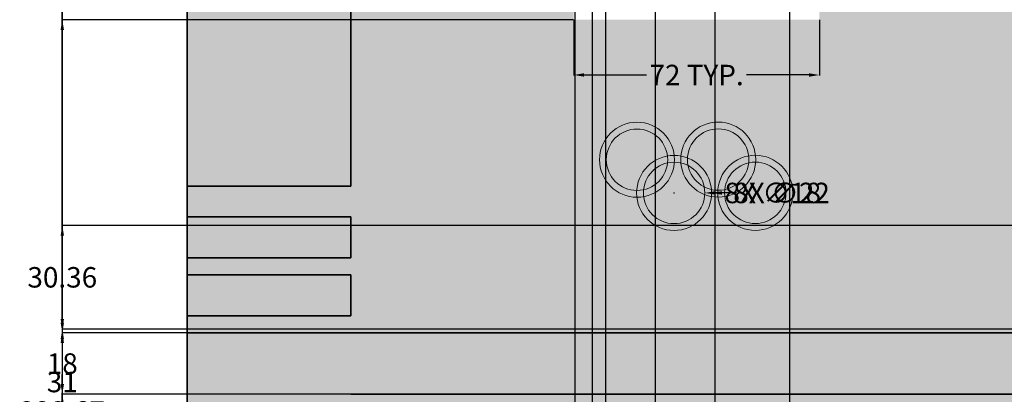
# Model space of a CAD drawing. Units: inches. Extents: x 126 to 726, y 86 to 888.
# Tile 7 of 13: x 137 to 426, y 546 to 655. Entities that reach past the tile are written whole.
import ezdxf

# ---------------------------------------------------------------- set-up
doc = ezdxf.new("R2010")
doc.units = ezdxf.units.IN
doc.header["$MEASUREMENT"] = 0
for name, color, linetype, lineweight in [('A-ANNO-DIMS', 2, 'Continuous', 18), ('A-ELEV', 7, 'Continuous', 35), ('A-ELEV-DECO', 7, 'Continuous', 18), ('A-ELEV-PATT', 8, 'Continuous', 13)]:
    doc.layers.add(name, color=color, linetype=linetype, lineweight=lineweight)
doc.styles.get("Standard").update_dxf_attribs({"font": 'arial.ttf'})
doc.dimstyles.get("Standard").update_dxf_attribs({"dimtxt": 6, "dimasz": 3, "dimexe": 0.18, "dimexo": 0.0625, "dimgap": 0.09, "dimtad": 0, "dimtih": 1, "dimtoh": 1, "dimdec": 0, "dimzin": 0, "dimdsep": 46, "dimlunit": 3, "dimtxsty": 'Standard', "dimcen": 0.09, "dimadec": 0, "dimazin": 0, "dimtfac": 1, "dimtdec": 0, "dimtofl": 0, "dimtmove": 0, "dimatfit": 3, "dimfxl": 1, "dimtolj": 1, "dimtzin": 0, "dimarcsym": 0})

# ---------------------------------------------------------------- blocks, each defined once
blk = doc.blocks.new('FACADE-STRIP')
for p, q in [((0, 0), (0, 12)), ((0, 12), (48, 12)), ((0, 0), (48, 0))]:
    blk.add_line(p, q)
blk = doc.blocks.new('MOTIF-RINGS')
for centre, radius in [((34.81, 20.77), 11), ((11, 20.74), 11), ((11, 20.74), 9), ((34.81, 20.77), 9), ((21.88, 11), 11), ((45.69, 11.03), 11), ((21.88, 11), 9), ((45.69, 11.03), 9)]:
    blk.add_circle(centre, radius)
blk = doc.blocks.new('*D6')
at = {"layer": 'A-ANNO-DIMS', "color": 0, "lineweight": -2, "transparency": 16777216}
for p, q in [((299.32, 655.29), (299.32, 638.97)), ((371.32, 655.29), (371.32, 638.97)), ((302.32, 639.15), (320.65, 639.15)), ((368.32, 639.15), (349.99, 639.15))]:
    blk.add_line(p, q, dxfattribs=at)
at = {"layer": 'A-ANNO-DIMS', "color": 0, "transparency": 16777216}
for points in [[(302.32, 639.65), (302.32, 638.65), (299.32, 639.15)], [(368.32, 639.65), (368.32, 638.65), (371.32, 639.15)]]:
    blk.add_solid(points, dxfattribs=at)
at = {"layer": 'Defpoints', "color": 0, "transparency": 16777216}
for p in [(299.32, 655.35), (371.32, 655.35), (371.32, 639.15)]:
    blk.add_point(p, dxfattribs=at)
at = {"layer": 'A-ANNO-DIMS', "color": 0, "transparency": 16777216, "insert": (335.32, 639.15), "char_height": 6, "attachment_point": 5}
blk.add_mtext('\\A1;72 TYP.', dxfattribs=at)
blk = doc.blocks.new('*D13')
at = {"layer": 'A-ANNO-DIMS', "color": 0, "lineweight": -2, "transparency": 16777216}
for p, q in [((665.97, 642.98), (665.97, 90.21)), ((185.97, 126.98), (185.97, 90.21)), ((188.97, 90.39), (419.15, 90.39)), ((662.97, 90.39), (432.8, 90.39))]:
    blk.add_line(p, q, dxfattribs=at)
at = {"layer": 'A-ANNO-DIMS', "color": 0, "transparency": 16777216}
for points in [[(188.97, 90.89), (188.97, 89.89), (185.97, 90.39)], [(662.97, 90.89), (662.97, 89.89), (665.97, 90.39)]]:
    blk.add_solid(points, dxfattribs=at)
at = {"layer": 'Defpoints', "color": 0, "transparency": 16777216}
for p in [(665.97, 643.04), (185.97, 127.04), (665.97, 90.39)]:
    blk.add_point(p, dxfattribs=at)
at = {"layer": 'A-ANNO-DIMS', "color": 0, "transparency": 16777216, "insert": (425.97, 90.39), "char_height": 6, "attachment_point": 5}
blk.add_mtext('\\A1;480', dxfattribs=at)
blk = doc.blocks.new('*D14')
at = {"layer": 'A-ANNO-DIMS', "color": 0, "lineweight": -2, "transparency": 16777216}
for p, q in [((185.91, 847.04), (149.14, 847.04)), ((149.32, 844.04), (149.32, 490.2)), ((149.32, 130.04), (149.32, 483.89)), ((185.91, 127.04), (149.14, 127.04))]:
    blk.add_line(p, q, dxfattribs=at)
at = {"layer": 'A-ANNO-DIMS', "color": 0, "transparency": 16777216}
for points in [[(148.82, 844.04), (149.82, 844.04), (149.32, 847.04)], [(148.82, 130.04), (149.82, 130.04), (149.32, 127.04)]]:
    blk.add_solid(points, dxfattribs=at)
at = {"layer": 'Defpoints', "color": 0, "transparency": 16777216}
for p in [(149.32, 847.04), (185.97, 847.04), (185.97, 127.04)]:
    blk.add_point(p, dxfattribs=at)
at = {"layer": 'A-ANNO-DIMS', "color": 0, "transparency": 16777216, "insert": (149.32, 487.04), "char_height": 6, "attachment_point": 5}
blk.add_mtext('\\A1;720', dxfattribs=at)
blk = doc.blocks.new('*D17')
at = {"layer": 'A-ANNO-DIMS', "color": 0, "lineweight": -2, "transparency": 16777216}
for p, q in [((299.26, 655.35), (149.14, 655.35)), ((149.32, 652.35), (149.32, 543.67)), ((149.32, 428.68), (149.32, 537.37)), ((299.6, 425.68), (149.14, 425.68))]:
    blk.add_line(p, q, dxfattribs=at)
at = {"layer": 'A-ANNO-DIMS', "color": 0, "transparency": 16777216}
for points in [[(148.82, 652.35), (149.82, 652.35), (149.32, 655.35)], [(148.82, 428.68), (149.82, 428.68), (149.32, 425.68)]]:
    blk.add_solid(points, dxfattribs=at)
at = {"layer": 'Defpoints', "color": 0, "transparency": 16777216}
for p in [(149.32, 655.35), (299.32, 655.35), (299.67, 425.68)]:
    blk.add_point(p, dxfattribs=at)
at = {"layer": 'A-ANNO-DIMS', "color": 0, "transparency": 16777216, "insert": (149.32, 540.52), "char_height": 6, "attachment_point": 5}
blk.add_mtext('\\A1;229.67', dxfattribs=at)
blk = doc.blocks.new('*D20')
at = {"layer": 'A-ANNO-DIMS', "color": 0, "lineweight": -2, "transparency": 16777216}
for p, q in [((233.91, 545.58), (149.14, 545.58)), ((149.32, 542.58), (149.32, 482.74)), ((149.32, 416.58), (149.32, 476.43)), ((233.91, 413.58), (149.14, 413.58))]:
    blk.add_line(p, q, dxfattribs=at)
at = {"layer": 'A-ANNO-DIMS', "color": 0, "transparency": 16777216}
for points in [[(148.82, 542.58), (149.82, 542.58), (149.32, 545.58)], [(148.82, 416.58), (149.82, 416.58), (149.32, 413.58)]]:
    blk.add_solid(points, dxfattribs=at)
at = {"layer": 'Defpoints', "color": 0, "transparency": 16777216}
for p in [(149.32, 545.58), (233.97, 545.58), (233.97, 413.58)]:
    blk.add_point(p, dxfattribs=at)
at = {"layer": 'A-ANNO-DIMS', "color": 0, "transparency": 16777216, "insert": (149.32, 479.58), "char_height": 6, "attachment_point": 5}
blk.add_mtext('\\A1;132', dxfattribs=at)
blk = doc.blocks.new('*D21')
at = {"layer": 'A-ANNO-DIMS', "color": 0, "lineweight": -2, "transparency": 16777216}
for p, q in [((431.28, 563.58), (149.14, 563.58)), ((149.32, 560.58), (149.32, 557.74)), ((149.32, 548.58), (149.32, 551.43)), ((233.91, 545.58), (149.14, 545.58))]:
    blk.add_line(p, q, dxfattribs=at)
at = {"layer": 'A-ANNO-DIMS', "color": 0, "transparency": 16777216}
for points in [[(148.82, 560.58), (149.82, 560.58), (149.32, 563.58)], [(148.82, 548.58), (149.82, 548.58), (149.32, 545.58)]]:
    blk.add_solid(points, dxfattribs=at)
at = {"layer": 'Defpoints', "color": 0, "transparency": 16777216}
for p in [(149.32, 563.58), (431.34, 563.58), (233.97, 545.58)]:
    blk.add_point(p, dxfattribs=at)
at = {"layer": 'A-ANNO-DIMS', "color": 0, "transparency": 16777216, "insert": (149.32, 554.58), "char_height": 6, "attachment_point": 5}
blk.add_mtext('\\A1;18', dxfattribs=at)
blk = doc.blocks.new('*D22')
at = {"layer": 'A-ANNO-DIMS', "color": 0, "lineweight": -2, "transparency": 16777216}
for p, q in [((185.91, 847.04), (149.14, 847.04)), ((149.32, 844.04), (149.32, 708.47)), ((149.32, 566.58), (149.32, 702.16)), ((431.28, 563.58), (149.14, 563.58))]:
    blk.add_line(p, q, dxfattribs=at)
at = {"layer": 'A-ANNO-DIMS', "color": 0, "transparency": 16777216}
for points in [[(148.82, 844.04), (149.82, 844.04), (149.32, 847.04)], [(148.82, 566.58), (149.82, 566.58), (149.32, 563.58)]]:
    blk.add_solid(points, dxfattribs=at)
at = {"layer": 'Defpoints', "color": 0, "transparency": 16777216}
for p in [(149.32, 847.04), (185.97, 847.04), (431.34, 563.58)]:
    blk.add_point(p, dxfattribs=at)
at = {"layer": 'A-ANNO-DIMS', "color": 0, "transparency": 16777216, "insert": (149.32, 705.31), "char_height": 6, "attachment_point": 5}
blk.add_mtext('\\A1;283.46', dxfattribs=at)
blk = doc.blocks.new('*D32')
at = {"layer": 'A-ANNO-DIMS', "color": 0, "lineweight": -2, "transparency": 16777216}
for p, q in [((299.67, 533.75), (299.67, 883.87)), ((302.67, 883.69), (305.67, 883.69)), ((308.67, 524.75), (308.67, 883.87)), ((308.67, 883.69), (311.67, 883.69))]:
    blk.add_line(p, q, dxfattribs=at)
at = {"layer": 'A-ANNO-DIMS', "color": 0, "transparency": 16777216}
for points in [[(302.67, 884.19), (302.67, 883.19), (299.67, 883.69)], [(305.67, 884.19), (305.67, 883.19), (308.67, 883.69)]]:
    blk.add_solid(points, dxfattribs=at)
at = {"layer": 'Defpoints', "color": 0, "transparency": 16777216}
for p in [(308.67, 883.69), (299.67, 533.68), (308.67, 524.68)]:
    blk.add_point(p, dxfattribs=at)
at = {"layer": 'A-ANNO-DIMS', "color": 0, "transparency": 16777216, "insert": (313.73, 883.69), "char_height": 6, "attachment_point": 5}
blk.add_mtext('\\A1;9', dxfattribs=at)
blk = doc.blocks.new('*D33')
at = {"layer": 'A-ANNO-DIMS', "color": 0, "lineweight": -2, "transparency": 16777216}
for p, q in [((308.67, 524.75), (308.67, 883.87)), ((311.67, 883.69), (331.29, 883.69)), ((359.67, 883.69), (340.04, 883.69)), ((362.67, 524.75), (362.67, 883.87))]:
    blk.add_line(p, q, dxfattribs=at)
at = {"layer": 'A-ANNO-DIMS', "color": 0, "transparency": 16777216}
for points in [[(311.67, 884.19), (311.67, 883.19), (308.67, 883.69)], [(359.67, 884.19), (359.67, 883.19), (362.67, 883.69)]]:
    blk.add_solid(points, dxfattribs=at)
at = {"layer": 'Defpoints', "color": 0, "transparency": 16777216}
for p in [(362.67, 883.69), (308.67, 524.68), (362.67, 524.68)]:
    blk.add_point(p, dxfattribs=at)
at = {"layer": 'A-ANNO-DIMS', "color": 0, "transparency": 16777216, "insert": (335.67, 883.69), "char_height": 6, "attachment_point": 5}
blk.add_mtext('\\A1;54', dxfattribs=at)
blk = doc.blocks.new('*D38')
at = {"layer": 'A-ANNO-DIMS', "color": 0, "lineweight": -2, "transparency": 16777216}
for p, q in [((304.8, 168.3), (304.8, 883.87)), ((307.8, 883.69), (320.3, 883.69)), ((323.3, 174.45), (323.3, 883.87)), ((323.3, 883.69), (326.3, 883.69))]:
    blk.add_line(p, q, dxfattribs=at)
at = {"layer": 'A-ANNO-DIMS', "color": 0, "transparency": 16777216}
for points in [[(307.8, 884.19), (307.8, 883.19), (304.8, 883.69)], [(320.3, 884.19), (320.3, 883.19), (323.3, 883.69)]]:
    blk.add_solid(points, dxfattribs=at)
at = {"layer": 'Defpoints', "color": 0, "transparency": 16777216}
for p in [(323.3, 883.69), (323.3, 174.39), (304.8, 168.24)]:
    blk.add_point(p, dxfattribs=at)
at = {"layer": 'A-ANNO-DIMS', "color": 0, "transparency": 16777216, "insert": (338.59, 883.69), "char_height": 6, "attachment_point": 5}
blk.add_mtext('\\A1;18.505', dxfattribs=at)
blk = doc.blocks.new('*D39')
at = {"layer": 'A-ANNO-DIMS', "color": 0, "lineweight": -2, "transparency": 16777216}
for p, q in [((323.3, 174.45), (323.3, 883.87)), ((326.3, 883.69), (337.74, 883.69)), ((340.74, 168.3), (340.74, 883.87)), ((340.74, 883.69), (343.74, 883.69))]:
    blk.add_line(p, q, dxfattribs=at)
at = {"layer": 'A-ANNO-DIMS', "color": 0, "transparency": 16777216}
for points in [[(326.3, 884.19), (326.3, 883.19), (323.3, 883.69)], [(337.74, 884.19), (337.74, 883.19), (340.74, 883.69)]]:
    blk.add_solid(points, dxfattribs=at)
at = {"layer": 'Defpoints', "color": 0, "transparency": 16777216}
for p in [(340.74, 883.69), (323.3, 174.39), (340.74, 168.24)]:
    blk.add_point(p, dxfattribs=at)
at = {"layer": 'A-ANNO-DIMS', "color": 0, "transparency": 16777216, "insert": (355.99, 883.69), "char_height": 6, "attachment_point": 5}
blk.add_mtext('\\A1;17.434', dxfattribs=at)
blk = doc.blocks.new('*D59')
at = {"layer": 'A-ANNO-DIMS', "color": 0, "lineweight": -2, "transparency": 16777216}
for p, q in [((485.91, 564.68), (149.14, 564.68)), ((149.32, 561.68), (149.32, 552.34)), ((149.32, 536.68), (149.32, 546.03)), ((485.91, 533.68), (149.14, 533.68))]:
    blk.add_line(p, q, dxfattribs=at)
at = {"layer": 'A-ANNO-DIMS', "color": 0, "transparency": 16777216}
for points in [[(148.82, 561.68), (149.82, 561.68), (149.32, 564.68)], [(148.82, 536.68), (149.82, 536.68), (149.32, 533.68)]]:
    blk.add_solid(points, dxfattribs=at)
at = {"layer": 'Defpoints', "color": 0, "transparency": 16777216}
for p in [(149.32, 564.68), (485.97, 564.68), (485.97, 533.68)]:
    blk.add_point(p, dxfattribs=at)
at = {"layer": 'A-ANNO-DIMS', "color": 0, "transparency": 16777216, "insert": (149.32, 549.18), "char_height": 6, "attachment_point": 5}
blk.add_mtext('\\A1;31', dxfattribs=at)
blk = doc.blocks.new('*D60')
at = {"layer": 'A-ANNO-DIMS', "color": 0, "lineweight": -2, "transparency": 16777216}
for p, q in [((485.91, 595.04), (149.14, 595.04)), ((149.32, 592.04), (149.32, 583.02)), ((149.32, 567.68), (149.32, 576.71)), ((485.91, 564.68), (149.14, 564.68))]:
    blk.add_line(p, q, dxfattribs=at)
at = {"layer": 'A-ANNO-DIMS', "color": 0, "transparency": 16777216}
for points in [[(148.82, 592.04), (149.82, 592.04), (149.32, 595.04)], [(148.82, 567.68), (149.82, 567.68), (149.32, 564.68)]]:
    blk.add_solid(points, dxfattribs=at)
at = {"layer": 'Defpoints', "color": 0, "transparency": 16777216}
for p in [(149.32, 595.04), (485.97, 595.04), (485.97, 564.68)]:
    blk.add_point(p, dxfattribs=at)
at = {"layer": 'A-ANNO-DIMS', "color": 0, "transparency": 16777216, "insert": (149.32, 579.86), "char_height": 6, "attachment_point": 5}
blk.add_mtext('\\A1;30.36', dxfattribs=at)
blk = doc.blocks.new('*D81')
at = {"layer": 'A-ANNO-DIMS', "color": 0, "lineweight": -2, "transparency": 16777216}
for p, q in [((328.63, 604.58), (328.81, 604.58)), ((328.72, 604.49), (328.72, 604.67)), ((346.32, 604.59), (342.72, 604.59))]:
    blk.add_line(p, q, dxfattribs=at)
at = {"layer": 'A-ANNO-DIMS', "color": 0, "transparency": 16777216}
blk.add_solid([(342.72, 605.09), (342.72, 604.09), (339.72, 604.59)], dxfattribs=at)
at = {"layer": 'Defpoints', "color": 0, "transparency": 16777216}
for p in [(317.72, 604.58), (339.72, 604.59)]:
    blk.add_point(p, dxfattribs=at)
at = {"layer": 'A-ANNO-DIMS', "color": 0, "transparency": 16777216, "insert": (360.23, 604.59), "char_height": 6, "attachment_point": 5}
blk.add_mtext('\\A1;8X ∅22', dxfattribs=at)
blk = doc.blocks.new('*D82')
at = {"layer": 'A-ANNO-DIMS', "color": 0, "lineweight": -2, "transparency": 16777216}
for p, q in [((328.63, 604.58), (328.81, 604.58)), ((328.72, 604.49), (328.72, 604.67)), ((343.72, 604.59), (340.72, 604.59))]:
    blk.add_line(p, q, dxfattribs=at)
at = {"layer": 'A-ANNO-DIMS', "color": 0, "transparency": 16777216}
blk.add_solid([(340.72, 605.09), (340.72, 604.09), (337.72, 604.59)], dxfattribs=at)
at = {"layer": 'Defpoints', "color": 0, "transparency": 16777216}
for p in [(319.72, 604.58), (337.72, 604.59)]:
    blk.add_point(p, dxfattribs=at)
at = {"layer": 'A-ANNO-DIMS', "color": 0, "transparency": 16777216, "insert": (357.67, 604.59), "char_height": 6, "attachment_point": 5}
blk.add_mtext('\\A1;8X ∅18', dxfattribs=at)

msp = doc.modelspace()

# ---------------------------------------------------------------- hatches: boundary and pattern name
at = {"layer": 'A-ELEV-PATT'}
h = msp.add_hatch(color=256, dxfattribs=at)
h.dxf.hatch_style = 1
h.paths.add_polyline_path([(233.9749, 545.5846), (431.3386, 545.5846), (431.3386, 563.5846), (185.9749, 563.5846), (185.9749, 395.5846), (431.3386, 395.5846), (431.3386, 413.5846), (233.9749, 413.5846)])
h.paths.add_polyline_path([(233.9749, 835.0424), (485.9749, 835.0424), (605.9749, 835.0424), (605.9749, 847.0424), (485.9749, 847.0424), (185.9749, 847.0424), (185.9749, 606.5846), (233.9749, 606.5846)])
h.paths.add_polyline_path([(233.9749, 597.5846), (185.9749, 597.5846), (185.9749, 585.5846), (233.9749, 585.5846)])
h.paths.add_polyline_path([(233.9749, 580.5846), (185.9749, 580.5846), (185.9749, 568.5846), (233.9749, 568.5846)])
h = msp.add_hatch(color=256, dxfattribs=at)
h.dxf.hatch_style = 1
h.paths.add_polyline_path([(437.9749, 499.1312), (485.9749, 499.1312), (485.9749, 501.4423), (437.9749, 501.4423), (437.9749, 513.4423), (485.9749, 513.4423), (485.9749, 515.7534), (437.9749, 515.7534), (437.9749, 527.7534), (485.9749, 527.7534), (485.9749, 530.0646), (437.9749, 530.0646), (437.9749, 542.0646), (485.9749, 542.0646), (485.9749, 544.3757), (437.9749, 544.3757), (437.9749, 556.3757), (485.9749, 556.3757), (485.9749, 558.6868), (437.9749, 558.6868), (437.9749, 570.6868), (485.9749, 570.6868), (485.9749, 572.9979), (437.9749, 572.9979), (437.9749, 584.9979), (485.9749, 584.9979), (485.9749, 587.309), (437.9749, 587.309), (437.9749, 595.0424), (429.9749, 595.0424), (429.9749, 607.0424), (437.9749, 607.0424), (437.9749, 615.9312), (437.9749, 630.2423), (437.9749, 642.2423), (485.9749, 642.2423), (485.9749, 644.5534), (437.9749, 644.5534), (437.9749, 656.5534), (485.9749, 656.5534), (485.9749, 658.8645), (437.9749, 658.8645), (437.9749, 670.8645), (485.9749, 670.8645), (485.9749, 673.1757), (437.9749, 673.1757), (437.9749, 685.1757), (485.9749, 685.1757), (485.9749, 687.4868), (437.9749, 687.4868), (437.9749, 699.4868), (485.9749, 699.4868), (485.9749, 701.7979), (437.9749, 701.7979), (437.9749, 713.7979), (485.9749, 713.7979), (485.9749, 716.109), (437.9749, 716.109), (437.9749, 728.109), (485.9749, 728.109), (485.9749, 730.4201), (437.9749, 730.4201), (437.9749, 742.4201), (485.9749, 742.4201), (485.9749, 744.7312), (437.9749, 744.7312), (437.9749, 756.7312), (485.9749, 756.7312), (485.9749, 759.0423), (437.9749, 759.0423), (437.9749, 771.0423), (485.9749, 771.0423), (485.9749, 773.3534), (437.9749, 773.3534), (437.9749, 785.3534), (485.9749, 785.3534), (485.9749, 787.6645), (437.9749, 787.6645), (437.9749, 799.6645), (485.9749, 799.6645), (485.9749, 801.9756), (437.9749, 801.9756), (437.9749, 811.2868), (485.9749, 811.2868), (485.9749, 813.9756), (437.9749, 813.9756), (437.9749, 825.9756), (485.9749, 825.9756), (485.9749, 835.0424), (233.9749, 835.0424), (233.9749, 606.5846), (185.9749, 606.5846), (185.9749, 597.5846), (233.9749, 597.5846), (233.9749, 585.5846), (185.9749, 585.5846), (185.9749, 580.5846), (233.9749, 580.5846), (233.9749, 568.5846), (185.9749, 568.5846), (185.9749, 563.5846), (431.3386, 563.5846), (431.3386, 545.5846), (233.9749, 545.5846), (233.9749, 413.5846), (431.3386, 413.5846), (431.3386, 395.5846), (185.9749, 395.5846), (185.9749, 386.5846), (233.9749, 386.5846), (233.9749, 374.5846), (185.9749, 374.5846), (185.9749, 369.5846), (233.9749, 369.5846), (233.9749, 357.5846), (185.9749, 357.5846), (185.9749, 352.5846), (233.9749, 352.5846), (233.9749, 340.5846), (185.9749, 340.5846), (185.9749, 331.5846), (233.9749, 331.5846), (233.9749, 127.0424), (485.9749, 127.0424), (485.9749, 129.3535), (437.9749, 129.3535), (437.9749, 141.3535), (485.9749, 141.3535), (485.9749, 143.6646), (437.9749, 143.6646), (437.9749, 155.6646), (485.9749, 155.6646), (485.9749, 157.9757), (437.9749, 157.9757), (437.9749, 169.9757), (485.9749, 169.9757), (485.9749, 172.2868), (437.9749, 172.2868), (437.9749, 184.2868), (485.9749, 184.2868), (485.9749, 186.5979), (437.9749, 186.5979), (437.9749, 198.5979), (485.9749, 198.5979), (485.9749, 200.909), (437.9749, 200.909), (437.9749, 212.909), (485.9749, 212.909), (485.9749, 215.2201), (437.9749, 215.2201), (437.9749, 227.2201), (485.9749, 227.2201), (485.9749, 229.5312), (437.9749, 229.5312), (437.9749, 241.5312), (485.9749, 241.5312), (485.9749, 243.8424), (437.9749, 243.8424), (437.9749, 255.8424), (485.9749, 255.8424), (485.9749, 258.1535), (437.9749, 258.1535), (437.9749, 270.1535), (485.9749, 270.1535), (485.9749, 272.4646), (437.9749, 272.4646), (437.9749, 284.4646), (485.9749, 284.4646), (485.9749, 286.7757), (437.9749, 286.7757), (437.9749, 298.7757), (485.9749, 298.7757), (485.9749, 301.0868), (437.9749, 301.0868), (437.9749, 313.0868), (485.9749, 313.0868), (485.9749, 315.3979), (437.9749, 315.3979), (437.9749, 327.3979), (485.9749, 327.3979), (485.9749, 329.709), (437.9749, 329.709), (437.9749, 341.709), (485.9749, 341.709), (485.9749, 344.0201), (437.9749, 344.0201), (437.9749, 355.0424), (429.9749, 355.0424), (429.9749, 367.0424), (437.9749, 367.0424), (437.9749, 372.6423), (437.9749, 386.9535), (437.9749, 401.2646), (437.9749, 413.2646), (485.9749, 413.2646), (485.9749, 415.5757), (437.9749, 415.5757), (437.9749, 427.5757), (485.9749, 427.5757), (485.9749, 429.8868), (437.9749, 429.8868), (437.9749, 441.8868), (485.9749, 441.8868), (485.9749, 444.1979), (437.9749, 444.1979), (437.9749, 456.1979), (485.9749, 456.1979), (485.9749, 458.509), (437.9749, 458.509), (437.9749, 470.509), (485.9749, 470.509), (485.9749, 472.8201), (437.9749, 472.8201), (437.9749, 484.8201), (485.9749, 484.8201), (485.9749, 487.1312), (437.9749, 487.1312)])
h.paths.add_polyline_path([(299.6658, 533.6845), (371.6658, 533.6845), (371.6658, 425.6845), (299.6658, 425.6845)], flags=16)
h.paths.add_polyline_path([(308.6658, 524.6845), (362.6658, 524.6845), (362.6658, 434.6845), (308.6658, 434.6845)], flags=0)
h.paths.add_polyline_path([(317.7956, 603.3211, -0.4129833), (306.8418, 614.321, -0.94403766), (328.769, 615.5845, -0.04423165), (330.7031, 615.4048, -0.89973713), (352.5798, 615.6161, -0.4129833), (363.5336, 604.6162, -0.94403766), (341.6064, 603.3528, -0.04423165), (339.6723, 603.5324, -0.89973713)], flags=16)
h.paths.add_polyline_path([(319.7228, 604.5846, -0.02633223), (319.7726, 605.5306, -0.47905713), (308.8418, 614.321, -1), (326.8418, 614.321, -0.02633223), (326.7919, 613.375, -0.17413188), (332.826, 612.5948, -0.04918553), (332.6526, 614.3527, -1), (350.6526, 614.3527, -0.02633223), (350.6028, 613.4067, -0.47905713), (361.5336, 604.6162, -1), (343.5336, 604.6162, -0.02633223), (343.5834, 605.5622, -0.17413188), (337.5494, 606.3424, -0.04918553), (337.7228, 604.5846, -1)], flags=0)
h.paths.add_polyline_path([(328.769, 355.6561, -0.04423165), (330.7031, 355.4765, -0.89973713), (352.5798, 355.6878, -0.4129833), (363.5336, 344.6879, -0.94403766), (341.6064, 343.4244, -0.04423165), (339.6723, 343.604, -0.89973713), (317.7956, 343.3927, -0.4129833), (306.8418, 354.3926, -0.94403766)], flags=16)
h.paths.add_polyline_path([(326.8418, 354.3926, -0.02633223), (326.7919, 353.4466, -0.17413188), (332.826, 352.6664, -0.04918553), (332.6526, 354.4243, -1), (350.6526, 354.4243, -0.02633223), (350.6028, 353.4783, -0.47905713), (361.5336, 344.6879, -1), (343.5336, 344.6879, -0.02633223), (343.5834, 345.6339, -0.17413188), (337.5494, 346.4141, -0.04918553), (337.7228, 344.6562, -1), (319.7228, 344.6562, -0.02633223), (319.7726, 345.6022, -0.47905713), (308.8418, 354.3926, -1)], flags=0)
h.paths.add_polyline_path([(299.3189, 655.3527), (299.3189, 763.3527), (371.3189, 763.3527), (371.3189, 655.3527)], flags=16)
h.paths.add_polyline_path([(308.3189, 664.3527), (308.3189, 754.3527), (362.3189, 754.3527), (362.3189, 664.3527)], flags=0)
h.paths.add_polyline_path([(299.6658, 303.5875), (371.6658, 303.5875), (371.6658, 195.5875), (299.6658, 195.5875)], flags=16)
h.paths.add_polyline_path([(308.6658, 294.5875), (362.6658, 294.5875), (362.6658, 204.5875), (308.6658, 204.5875)], flags=0)
h.paths.add_polyline_path([(326.3038, 177.3867), (346.055, 177.3867, -0.41421356), (349.055, 174.3867), (349.055, 171.2378), (363.489, 171.2378, -0.41421356), (366.489, 168.2378), (366.489, 159.7133, -0.41421356), (363.489, 156.7133), (343.7379, 156.7133, -0.41421356), (340.7379, 159.7133), (340.7379, 162.8622), (330.5504, 162.8622), (330.5504, 159.7133, -0.41421356), (327.5504, 156.7133), (307.7992, 156.7133, -0.41421356), (304.7992, 159.7133), (304.7992, 168.2378, -0.41421356), (307.7992, 171.2378), (323.3038, 171.2378), (323.3038, 174.3867, -0.41421356)], flags=16)
h.paths.add_polyline_path([(326.3038, 175.3867), (346.055, 175.3867, -0.41421356), (347.055, 174.3867), (347.055, 169.2378), (363.489, 169.2378, -0.41421356), (364.489, 168.2378), (364.489, 159.7133, -0.41421356), (363.489, 158.7133), (343.7379, 158.7133, -0.41421356), (342.7379, 159.7133), (342.7379, 164.8622), (328.5504, 164.8622), (328.5504, 159.7133, -0.41421356), (327.5504, 158.7133), (307.7992, 158.7133, -0.41421356), (306.7992, 159.7133), (306.7992, 168.2378, -0.41421356), (307.7992, 169.2378), (325.3038, 169.2378), (325.3038, 174.3867, -0.41421356)], flags=0)
h = msp.add_hatch(dxfattribs=at)
h.set_pattern_fill('GRAVEL', color=256, scale=40)
h.paths.add_polyline_path([(437.9749, 642.2423), (485.9749, 642.2423), (485.9749, 644.5534), (437.9749, 644.5534), (437.9749, 656.5534), (485.9749, 656.5534), (485.9749, 658.8645), (437.9749, 658.8645), (437.9749, 670.8645), (485.9749, 670.8645), (485.9749, 673.1757), (437.9749, 673.1757), (437.9749, 685.1757), (485.9749, 685.1757), (485.9749, 687.4868), (437.9749, 687.4868), (437.9749, 699.4868), (485.9749, 699.4868), (485.9749, 701.7979), (437.9749, 701.7979), (437.9749, 713.7979), (485.9749, 713.7979), (485.9749, 716.109), (437.9749, 716.109), (437.9749, 728.109), (485.9749, 728.109), (485.9749, 730.4201), (437.9749, 730.4201), (437.9749, 742.4201), (485.9749, 742.4201), (485.9749, 744.7312), (437.9749, 744.7312), (437.9749, 756.7312), (485.9749, 756.7312), (485.9749, 759.0423), (437.9749, 759.0423), (437.9749, 771.0423), (485.9749, 771.0423), (485.9749, 773.3534), (437.9749, 773.3534), (437.9749, 785.3534), (485.9749, 785.3534), (485.9749, 787.6645), (437.9749, 787.6645), (437.9749, 799.6645), (485.9749, 799.6645), (485.9749, 801.9756), (437.9749, 801.9756), (437.9749, 811.2868), (485.9749, 811.2868), (485.9749, 813.9756), (437.9749, 813.9756), (437.9749, 825.9756), (485.9749, 825.9756), (485.9749, 835.0424), (233.9749, 835.0424), (233.9749, 606.5846), (185.9749, 606.5846), (185.9749, 597.5846), (233.9749, 597.5846), (233.9749, 585.5846), (185.9749, 585.5846), (185.9749, 580.5846), (233.9749, 580.5846), (233.9749, 568.5846), (185.9749, 568.5846), (185.9749, 563.5846), (431.3386, 563.5846), (431.3386, 545.5846), (233.9749, 545.5846), (233.9749, 413.5846), (431.3386, 413.5846), (431.3386, 395.5846), (185.9749, 395.5846), (185.9749, 386.5846), (233.9749, 386.5846), (233.9749, 374.5846), (185.9749, 374.5846), (185.9749, 369.5846), (233.9749, 369.5846), (233.9749, 357.5846), (185.9749, 357.5846), (185.9749, 352.5846), (233.9749, 352.5846), (233.9749, 340.5846), (185.9749, 340.5846), (185.9749, 331.5846), (233.9749, 331.5846), (233.9749, 127.0424), (485.9749, 127.0424), (485.9749, 129.3535), (437.9749, 129.3535), (437.9749, 141.3535), (485.9749, 141.3535), (485.9749, 143.6646), (437.9749, 143.6646), (437.9749, 155.6646), (485.9749, 155.6646), (485.9749, 157.9757), (437.9749, 157.9757), (437.9749, 169.9757), (485.9749, 169.9757), (485.9749, 172.2868), (437.9749, 172.2868), (437.9749, 184.2868), (485.9749, 184.2868), (485.9749, 186.5979), (437.9749, 186.5979), (437.9749, 198.5979), (485.9749, 198.5979), (485.9749, 200.909), (437.9749, 200.909), (437.9749, 212.909), (485.9749, 212.909), (485.9749, 215.2201), (437.9749, 215.2201), (437.9749, 227.2201), (485.9749, 227.2201), (485.9749, 229.5312), (437.9749, 229.5312), (437.9749, 241.5312), (485.9749, 241.5312), (485.9749, 243.8424), (437.9749, 243.8424), (437.9749, 255.8424), (485.9749, 255.8424), (485.9749, 258.1535), (437.9749, 258.1535), (437.9749, 270.1535), (485.9749, 270.1535), (485.9749, 272.4646), (437.9749, 272.4646), (437.9749, 284.4646), (485.9749, 284.4646), (485.9749, 286.7757), (437.9749, 286.7757), (437.9749, 298.7757), (485.9749, 298.7757), (485.9749, 301.0868), (437.9749, 301.0868), (437.9749, 313.0868), (485.9749, 313.0868), (485.9749, 315.3979), (437.9749, 315.3979), (437.9749, 327.3979), (485.9749, 327.3979), (485.9749, 329.709), (437.9749, 329.709), (437.9749, 341.709), (485.9749, 341.709), (485.9749, 344.0201), (437.9749, 344.0201), (437.9749, 355.0424), (429.9749, 355.0424), (429.9749, 367.0424), (437.9749, 367.0424), (437.9749, 372.6423), (437.9749, 386.9535), (437.9749, 401.2646), (437.9749, 413.2646), (485.9749, 413.2646), (485.9749, 415.5757), (437.9749, 415.5757), (437.9749, 427.5757), (485.9749, 427.5757), (485.9749, 429.8868), (437.9749, 429.8868), (437.9749, 441.8868), (485.9749, 441.8868), (485.9749, 444.1979), (437.9749, 444.1979), (437.9749, 456.1979), (485.9749, 456.1979), (485.9749, 458.509), (437.9749, 458.509), (437.9749, 470.509), (485.9749, 470.509), (485.9749, 472.8201), (437.9749, 472.8201), (437.9749, 484.8201), (485.9749, 484.8201), (485.9749, 487.1312), (437.9749, 487.1312), (437.9749, 499.1312), (485.9749, 499.1312), (485.9749, 501.4423), (437.9749, 501.4423), (437.9749, 513.4423), (485.9749, 513.4423), (485.9749, 515.7534), (437.9749, 515.7534), (437.9749, 527.7534), (485.9749, 527.7534), (485.9749, 530.0646), (437.9749, 530.0646), (437.9749, 542.0646), (485.9749, 542.0646), (485.9749, 544.3757), (437.9749, 544.3757), (437.9749, 556.3757), (485.9749, 556.3757), (485.9749, 558.6868), (437.9749, 558.6868), (437.9749, 570.6868), (485.9749, 570.6868), (485.9749, 572.9979), (437.9749, 572.9979), (437.9749, 584.9979), (485.9749, 584.9979), (485.9749, 587.309), (437.9749, 587.309), (437.9749, 595.0424), (429.9749, 595.0424), (429.9749, 607.0424), (437.9749, 607.0424), (437.9749, 615.9312), (437.9749, 630.2423)])
h.paths.add_polyline_path([(371.3189, 655.3527), (299.3189, 655.3527), (299.3189, 763.3527), (371.3189, 763.3527)], flags=16)
h.paths.add_polyline_path([(363.5336, 604.6162, -0.94403766), (341.6064, 603.3528, -0.04423165), (339.6723, 603.5324, -0.89973713), (317.7956, 603.3211, -0.4129833), (306.8418, 614.321, -0.94403766), (328.769, 615.5845, -0.04423165), (330.7031, 615.4048, -0.89973713), (352.5798, 615.6161, -0.4129833)], flags=16)
h.paths.add_polyline_path([(361.5336, 604.6162, -1), (343.5336, 604.6162, -0.02633223), (343.5834, 605.5622, -0.17413188), (337.5494, 606.3424, -0.04918553), (337.7228, 604.5846, -1), (319.7228, 604.5846, -0.02633223), (319.7726, 605.5306, -0.47905713), (308.8418, 614.321, -1), (326.8418, 614.321, -0.02633223), (326.7919, 613.375, -0.17413188), (332.826, 612.5948, -0.04918553), (332.6526, 614.3527, -1), (350.6526, 614.3527, -0.02633223), (350.6028, 613.4067, -0.47905713)], flags=0)
h.paths.add_polyline_path([(362.3189, 664.3527), (308.3189, 664.3527), (308.3189, 754.3527), (362.3189, 754.3527)], flags=0)
h.paths.add_polyline_path([(371.6658, 533.6845), (371.6658, 425.6845), (299.6658, 425.6845), (299.6658, 533.6845)], flags=16)
h.paths.add_polyline_path([(362.6658, 524.6845), (362.6658, 434.6845), (308.6658, 434.6845), (308.6658, 524.6845)], flags=0)
h.paths.add_polyline_path([(352.5798, 355.6878, -0.4129833), (363.5336, 344.6879, -0.94403766), (341.6064, 343.4244, -0.04423165), (339.6723, 343.604, -0.89973713), (317.7956, 343.3927, -0.4129833), (306.8418, 354.3926, -0.94403766), (328.769, 355.6561, -0.04423165), (330.7031, 355.4765, -0.89973713)], flags=16)
h.paths.add_polyline_path([(350.6526, 354.4243, -0.02633223), (350.6028, 353.4783, -0.47905713), (361.5336, 344.6879, -1), (343.5336, 344.6879, -0.02633223), (343.5834, 345.6339, -0.17413188), (337.5494, 346.4141, -0.04918553), (337.7228, 344.6562, -1), (319.7228, 344.6562, -0.02633223), (319.7726, 345.6022, -0.47905713), (308.8418, 354.3926, -1), (326.8418, 354.3926, -0.02633223), (326.7919, 353.4466, -0.17413188), (332.826, 352.6664, -0.04918553), (332.6526, 354.4243, -1)], flags=0)
h.paths.add_polyline_path([(371.6658, 303.5875), (371.6658, 195.5875), (299.6658, 195.5875), (299.6658, 303.5875)], flags=16)
h.paths.add_polyline_path([(362.6658, 294.5875), (362.6658, 204.5875), (308.6658, 204.5875), (308.6658, 294.5875)], flags=0)
h.paths.add_polyline_path([(346.055, 177.3867, -0.41421356), (349.055, 174.3867), (349.055, 171.2378), (363.489, 171.2378, -0.41421356), (366.489, 168.2378), (366.489, 159.7133, -0.41421356), (363.489, 156.7133), (343.7379, 156.7133, -0.41421356), (340.7379, 159.7133), (340.7379, 162.8622), (330.5504, 162.8622), (330.5504, 159.7133, -0.41421356), (327.5504, 156.7133), (307.7992, 156.7133, -0.41421356), (304.7992, 159.7133), (304.7992, 168.2378, -0.41421356), (307.7992, 171.2378), (323.3038, 171.2378), (323.3038, 174.3867, -0.41421356), (326.3038, 177.3867)], flags=16)
h.paths.add_polyline_path([(346.055, 175.3867, -0.41421356), (347.055, 174.3867), (347.055, 169.2378), (363.489, 169.2378, -0.41421356), (364.489, 168.2378), (364.489, 159.7133, -0.41421356), (363.489, 158.7133), (343.7379, 158.7133, -0.41421356), (342.7379, 159.7133), (342.7379, 164.8622), (328.5504, 164.8622), (328.5504, 159.7133, -0.41421356), (327.5504, 158.7133), (307.7992, 158.7133, -0.41421356), (306.7992, 159.7133), (306.7992, 168.2378, -0.41421356), (307.7992, 169.2378), (325.3038, 169.2378), (325.3038, 174.3867, -0.41421356), (326.3038, 175.3867)], flags=0)
h = msp.add_hatch(color=256, dxfattribs=at)
h.dxf.hatch_style = 1
h.paths.add_polyline_path([(306.8418, 614.321, 0.4129833), (317.7956, 603.3211, -0.02878665), (317.7228, 604.5846, -0.0167625), (317.7475, 605.3215, -0.4111475), (308.8418, 614.321, -0.94107412), (326.7756, 615.4109, -0.04557115), (328.769, 615.5845, 0.94403766)])
h.paths.add_polyline_path([(350.5864, 615.4425, -0.04557115), (352.5798, 615.6161, 0.89973713), (330.7031, 615.4048, -0.04645219), (332.6665, 614.8533, -0.91517696)])
h.paths.add_polyline_path([(352.5798, 615.6161, -0.02878665), (352.6526, 614.3527, -0.0167625), (352.6279, 613.6157, -0.4111475), (361.5336, 604.6162, -0.94107412), (343.5998, 603.5264, -0.04557115), (341.6064, 603.3528, 0.94403766), (363.5336, 604.6162, 0.4129833)])
h.paths.add_polyline_path([(350.6028, 613.4067, 0.02633223), (350.6526, 614.3527, 0.03035736), (350.5864, 615.4425, 0.34414474), (341.5583, 605.3532, 0.05673494), (343.5834, 605.5622, -0.32288595)])
h.paths.add_polyline_path([(352.6279, 613.6157, 0.05673494), (350.6028, 613.4067, -0.32288595), (343.5834, 605.5622, 0.02633223), (343.5336, 604.6162, 0.03035736), (343.5998, 603.5264, 0.34414474)], flags=17)
h.paths.add_polyline_path([(332.6665, 614.8533, 0.01391386), (332.6526, 614.3527, 0.04918553), (332.826, 612.5948, -0.22909031), (337.5494, 606.3424, 0.0631426), (339.6784, 605.5719, 0.28599337)])
h.paths.add_polyline_path([(332.826, 612.5948, 0.0631426), (330.697, 613.3654, 0.28599337), (337.7088, 604.084, 0.01391386), (337.7228, 604.5846, 0.04918553), (337.5494, 606.3424, -0.22909031)])
h.paths.add_polyline_path([(328.8171, 613.5841, 0.05673494), (326.7919, 613.375, -0.32288595), (319.7726, 605.5306, 0.02633223), (319.7228, 604.5846, 0.03035736), (319.789, 603.4947, 0.34414474)])
h.paths.add_polyline_path([(326.7919, 613.375, 0.02633223), (326.8418, 614.321, 0.03035736), (326.7756, 615.4109, 0.34414474), (317.7475, 605.3215, 0.05673494), (319.7726, 605.5306, -0.32288595)], flags=17)
h.paths.add_polyline_path([(339.6723, 603.5324, -0.04645219), (337.7088, 604.084, -0.91517696), (319.789, 603.4947, -0.04557115), (317.7956, 603.3211, 0.89973713)])
h.paths.add_polyline_path([(341.5336, 604.6162, -0.0167625), (341.5583, 605.3532, -0.05271891), (339.6784, 605.5719, -0.022473), (339.7228, 604.5846, -0.02395419), (339.6723, 603.5324, 0.04423165), (341.6064, 603.3528, -0.02878665)])
h.paths.add_polyline_path([(339.6784, 605.5719, -0.0631426), (337.5494, 606.3424, -0.04918553), (337.7228, 604.5846, -0.01391386), (337.7088, 604.084, 0.04645219), (339.6723, 603.5324, 0.02395419), (339.7228, 604.5846, 0.022473)])
h.paths.add_polyline_path([(343.5336, 604.6162, -0.02633223), (343.5834, 605.5622, -0.05673494), (341.5583, 605.3532, 0.0167625), (341.5336, 604.6162, 0.02878665), (341.6064, 603.3528, 0.04557115), (343.5998, 603.5264, -0.03035736)])
h.paths.add_polyline_path([(352.6526, 614.3527, 0.02878665), (352.5798, 615.6161, 0.04557115), (350.5864, 615.4425, -0.03035736), (350.6526, 614.3527, -0.02633223), (350.6028, 613.4067, -0.05673494), (352.6279, 613.6157, 0.0167625)])
h.paths.add_polyline_path([(330.6526, 614.3527, -0.02395419), (330.7031, 615.4048, 0.04423165), (328.769, 615.5845, -0.02878665), (328.8418, 614.321, -0.0167625), (328.8171, 613.5841, -0.05271891), (330.697, 613.3654, -0.022473)])
h.paths.add_polyline_path([(332.6526, 614.3527, -0.01391386), (332.6665, 614.8533, 0.04645219), (330.7031, 615.4048, 0.02395419), (330.6526, 614.3527, 0.022473), (330.697, 613.3654, -0.0631426), (332.826, 612.5948, -0.04918553)])
h.paths.add_polyline_path([(328.769, 615.5845, 0.04557115), (326.7756, 615.4109, -0.03035736), (326.8418, 614.321, -0.02633223), (326.7919, 613.375, -0.05673494), (328.8171, 613.5841, 0.0167625), (328.8418, 614.321, 0.02878665)])
h.paths.add_polyline_path([(319.7228, 604.5846, -0.02633223), (319.7726, 605.5306, -0.05673494), (317.7475, 605.3215, 0.0167625), (317.7228, 604.5846, 0.02878665), (317.7956, 603.3211, 0.04557115), (319.789, 603.4947, -0.03035736)])
h = msp.add_hatch(color=256, dxfattribs=at)
h.dxf.hatch_style = 1
h.paths.add_polyline_path([(343.7379, 171.2378), (347.055, 171.2378), (347.055, 174.3867, 0.41421356), (346.055, 175.3867), (326.3038, 175.3867, 0.41421356), (325.3038, 174.3867), (325.3038, 171.2378), (327.5504, 171.2378, -0.41421356), (330.5504, 168.2378), (330.5504, 164.8622), (340.7379, 164.8622), (340.7379, 168.2378, -0.41421356)])
h.paths.add_polyline_path([(328.5504, 162.8622), (326.3038, 162.8622, -0.41421356), (323.3038, 165.8622), (323.3038, 169.2378), (307.7992, 169.2378, 0.41421356), (306.7992, 168.2378), (306.7992, 159.7133, 0.41421356), (307.7992, 158.7133), (327.5504, 158.7133, 0.41421356), (328.5504, 159.7133)])
h.paths.add_polyline_path([(328.5504, 168.2378, 0.41421356), (327.5504, 169.2378), (325.3038, 169.2378), (325.3038, 165.8622, 0.41421356), (326.3038, 164.8622), (328.5504, 164.8622)], flags=17)
h.paths.add_polyline_path([(364.489, 168.2378, 0.41421356), (363.489, 169.2378), (349.055, 169.2378), (349.055, 165.8622, -0.41421356), (346.055, 162.8622), (342.7379, 162.8622), (342.7379, 159.7133, 0.41421356), (343.7379, 158.7133), (363.489, 158.7133, 0.41421356), (364.489, 159.7133)])
h.paths.add_polyline_path([(347.055, 169.2378), (343.7379, 169.2378, 0.41421356), (342.7379, 168.2378), (342.7379, 164.8622), (346.055, 164.8622, 0.41421356), (347.055, 165.8622)], flags=17)
h.paths.add_polyline_path([(361.5336, 344.6879, 0.4111475), (352.6279, 353.6874, -0.34414474), (343.5998, 343.598, 0.94107412)])
h.paths.add_polyline_path([(332.6665, 354.9249, -0.28599337), (339.6784, 345.6435, 0.05271891), (341.5583, 345.4248, -0.34414474), (350.5864, 355.5141, 0.91517696)])
h.paths.add_polyline_path([(308.8418, 354.3926, 0.4111475), (317.7475, 345.3931, -0.34414474), (326.7756, 355.4825, 0.94107412)])
h.paths.add_polyline_path([(326.7919, 353.4466, 0.32288595), (319.7726, 345.6022, 0.32288595)])
h.paths.add_polyline_path([(330.697, 353.437, 0.05271891), (328.8171, 353.6557, -0.34414474), (319.789, 343.5663, 0.91517696), (337.7088, 344.1556, -0.28599337)])
h.paths.add_polyline_path([(332.826, 352.6664, 0.22909031), (337.5494, 346.4141, 0.22909031)], flags=17)
h.paths.add_polyline_path([(350.6028, 353.4783, 0.32288595), (343.5834, 345.6339, 0.32288595)])
h.paths.add_polyline_path([(332.6665, 614.8533, -0.28599337), (339.6784, 605.5719, 0.05271891), (341.5583, 605.3532, -0.34414474), (350.5864, 615.4425, 0.91517696)])
h.paths.add_polyline_path([(308.8418, 614.321, 0.4111475), (317.7475, 605.3215, -0.34414474), (326.7756, 615.4109, 0.94107412)])
h.paths.add_polyline_path([(337.7088, 604.084, -0.28599337), (330.697, 613.3654, 0.05271891), (328.8171, 613.5841, -0.34414474), (319.789, 603.4947, 0.91517696)])
h.paths.add_polyline_path([(361.5336, 604.6162, 0.4111475), (352.6279, 613.6157, -0.34414474), (343.5998, 603.5264, 0.94107412)])
h.paths.add_polyline_path([(350.6028, 613.4067, 0.32288595), (343.5834, 605.5622, 0.32288595)])
h.paths.add_polyline_path([(332.826, 612.5948, 0.22909031), (337.5494, 606.3424, 0.22909031)], flags=17)
h.paths.add_polyline_path([(326.7919, 613.375, 0.32288595), (319.7726, 605.5306, 0.32288595)])

# ---------------------------------------------------------------- linework, layer by layer
at = {"layer": 'A-ELEV'}
for p, q in [((185.9749, 847.0424), (185.9749, 127.0424)), ((233.9749, 835.0424), (233.9749, 606.5846)), ((233.9749, 606.5846), (185.9749, 606.5846)), ((431.3386, 563.5846), (185.9749, 563.5846)), ((431.3386, 545.5846), (233.9749, 545.5846))]:
    msp.add_line(p, q, dxfattribs=at)

# ---------------------------------------------------------------- block references
at = {"layer": 'A-ELEV', "rotation": 180}
for p in [(233.9748, 597.585), (233.9748, 580.585)]:
    msp.add_blockref('FACADE-STRIP', p, dxfattribs=at)
at = {"layer": 'A-ELEV-DECO'}
msp.add_blockref('MOTIF-RINGS', (306.842, 593.585), dxfattribs=at)

# ---------------------------------------------------------------- dimensions: what is measured, and where the dimension line sits
at = {"layer": 'A-ANNO-DIMS'}
for base, p1, p2, override, picture, middle in [((308.6658, 883.6924), (299.6658, 533.6845), (308.6658, 524.6845), {"dimdec": 0, "dimlfac": 1, "dimrnd": 0, "dimzin": 0, "dimdsep": 46, "dimlunit": 2}, '*D32', (313.7286, 883.6924)), ((323.3038, 883.6924), (304.7992, 168.2378), (323.3038, 174.3867), {"dimdec": 3, "dimlfac": 1, "dimrnd": 0, "dimzin": 0, "dimdsep": 46, "dimlunit": 2}, '*D38', (338.5882, 883.6924)), ((362.6658, 883.6924), (308.6658, 524.6845), (362.6658, 524.6845), {"dimdec": 0, "dimlfac": 1, "dimrnd": 0, "dimzin": 0, "dimdsep": 46, "dimlunit": 2}, '*D33', (335.6658, 883.6924)), ((340.7379, 883.6924), (323.3038, 174.3867), (340.7379, 168.2378), {"dimdec": 3, "dimlfac": 1, "dimrnd": 0, "dimzin": 0, "dimdsep": 46, "dimlunit": 2}, '*D39', (355.9875, 883.6924)), ((665.9749, 90.3924), (185.9749, 127.0424), (665.9749, 643.0424), {"dimdec": 0, "dimlfac": 1, "dimrnd": 0, "dimzin": 0, "dimdsep": 46, "dimlunit": 2}, '*D13', (425.9749, 90.3924))]:
    dim = msp.add_linear_dim(base=base, p1=p1, p2=p2, dimstyle='Standard', override=override, dxfattribs=at)
    dim.commit()
    dim.dimension.update_dxf_attribs({"geometry": picture, "text_midpoint": middle})
for base, p1, p2, override, picture, middle in [((149.3249, 847.0424), (431.3386, 563.5846), (185.9749, 847.0424), {"dimdec": 2, "dimlfac": 1, "dimrnd": 0, "dimzin": 0, "dimdsep": 46, "dimlunit": 2}, '*D22', (149.3249, 705.3135)), ((149.3249, 847.0424), (185.9749, 127.0424), (185.9749, 847.0424), {"dimdec": 0, "dimlfac": 1, "dimrnd": 0, "dimzin": 0, "dimdsep": 46, "dimlunit": 2}, '*D14', (149.3249, 487.0424)), ((149.3249, 655.3527), (299.6658, 425.6845), (299.3189, 655.3527), {"dimdec": 2, "dimlfac": 1, "dimrnd": 0, "dimzin": 0, "dimdsep": 46, "dimlunit": 2}, '*D17', (149.3249, 540.5186)), ((149.3249, 595.0424), (485.9749, 564.6845), (485.9749, 595.0424), {"dimdec": 2, "dimlfac": 1, "dimrnd": 0, "dimzin": 0, "dimdsep": 46, "dimlunit": 2}, '*D60', (149.3249, 579.8634)), ((149.3249, 564.6845), (485.9749, 533.6845), (485.9749, 564.6845), {"dimdec": 0, "dimlfac": 1, "dimrnd": 0, "dimzin": 0, "dimdsep": 46, "dimlunit": 2}, '*D59', (149.3249, 549.1845)), ((149.3249, 563.5846), (233.9749, 545.5846), (431.3386, 563.5846), {"dimdec": 0, "dimlfac": 1, "dimrnd": 0, "dimzin": 0, "dimdsep": 46, "dimlunit": 2}, '*D21', (149.3249, 554.5846)), ((149.3249, 545.5846), (233.9749, 413.5846), (233.9749, 545.5846), {"dimdec": 0, "dimlfac": 1, "dimrnd": 0, "dimzin": 0, "dimdsep": 46, "dimlunit": 2}, '*D20', (149.3249, 479.5846))]:
    dim = msp.add_linear_dim(base=base, p1=p1, p2=p2, angle=90, dimstyle='Standard', override=override, dxfattribs=at)
    dim.commit()
    dim.dimension.update_dxf_attribs({"geometry": picture, "text_midpoint": middle})
dim = msp.add_linear_dim(base=(371.3189, 639.1527), p1=(299.3189, 655.3527), p2=(371.3189, 655.3527), text='<> TYP.', dimstyle='Standard', override={"dimdec": 0, "dimlfac": 1, "dimrnd": 0, "dimzin": 0, "dimdsep": 46, "dimlunit": 2}, dxfattribs=at)
dim.commit()
dim.dimension.update_dxf_attribs({"geometry": '*D6', "text_midpoint": (335.3189, 639.1527)})
for p1, p2, picture, middle in [((317.7228, 604.5841), (339.7228, 604.585), '*D81', (346.3228, 604.5853)), ((319.7228, 604.5841), (337.7228, 604.585), '*D82', (343.7228, 604.5853))]:
    dim = msp.add_diameter_dim_2p(p1=p1, p2=p2, text='8X <>', dimstyle='Standard', override={"dimdec": 0, "dimlfac": 1, "dimrnd": 0, "dimzin": 0, "dimdsep": 46, "dimlunit": 2}, dxfattribs=at)
    dim.commit()
    dim.dimension.update_dxf_attribs({"geometry": picture, "text_midpoint": middle, "dimtype": 163})

doc.saveas('drawing.dxf')
